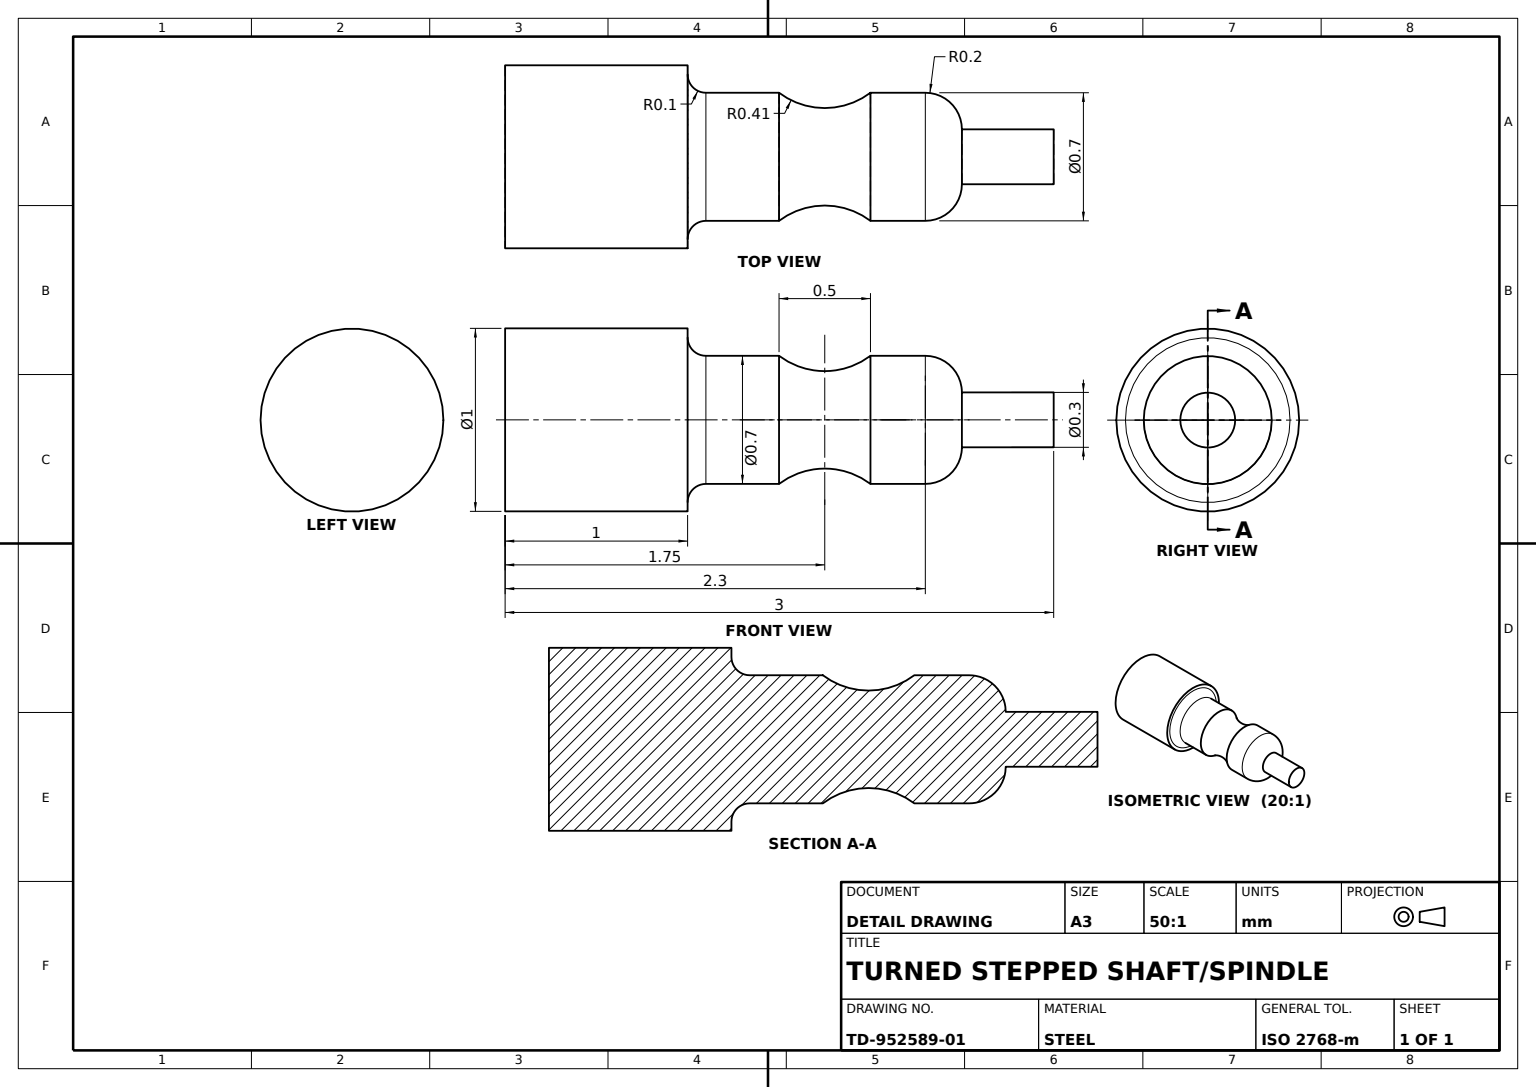
SolidWorks part; units mm, degrees
material "Plain Carbon Steel"
ref_plane "Front Plane" through (0, 0, 0) normal (0, 0, 1) x (1, 0, 0)
ref_plane "Top Plane" through (0, 0, 0) normal (0, 1, 0) x (1, 0, 0)
ref_plane "Right Plane" through (0, 0, 0) normal (1, 0, 0) x (0, 0, -1)
sketch "Pin Profile Sketch" plane through (0, 0, 0) normal (0, 0, 1) x (1, 0, 0)
  line L1 (3, 0) -> (3, -0.15)
  line L2 (3, -0.15) -> (2.498, -0.15)
  line L7 (2.298, -0.35) -> (1.998, -0.35)
  line L9 (1.498, -0.35) -> (1.098, -0.35)
  line L10 (0.998, -0.45) -> (0.998, -0.5)
  line L11 (0.998, -0.5) -> (0, -0.5)
  line L12 (0, -0.5) -> (0, 0)
  line L13 (0, 0) -> (3, 0)
  arc A1 (1.998, -0.35) -> (1.498, -0.35) centre (1.748, -0.6812) ccw
  arc A2 (1.098, -0.35) -> (0.998, -0.45) centre (1.098, -0.45) ccw
  arc A3 (2.298, -0.35) -> (2.498, -0.15) centre (2.298, -0.15) ccw
  dimension "D2" = 0.15
  dimension "D3" = 0.35
  dimension "D4" = 0.415
  dimension "D11" = 0.1
  dimension "D12" = 2.298
  dimension "D10" = 0.2
  dimension "D1" = 3
  dimension "D5" = 0.5
  dimension "D6" = 0.998
  dimension "D7" = 0.35
  dimension "D8" = 1.748
  dimension "D9" = 0.6812
revolve "Stepped Pin Revolve" add sketch "Pin Profile Sketch" angle 360 about L13
